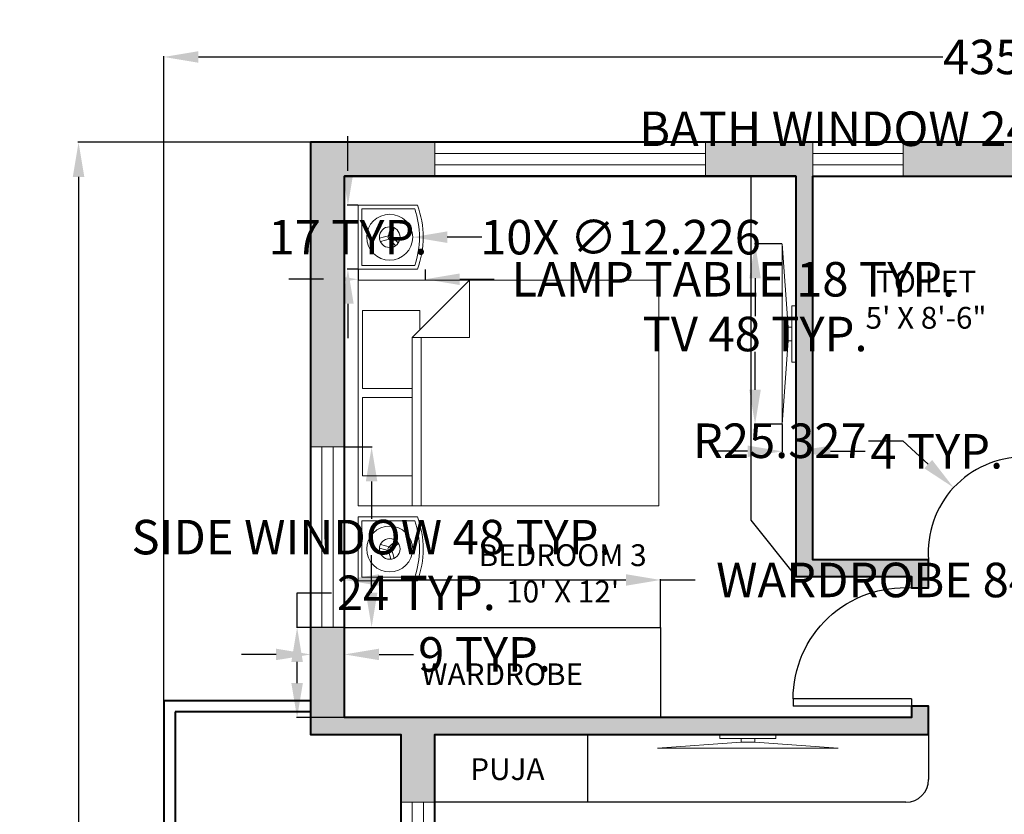
# Model space of a CAD drawing. Units: inches. Extents: x -51 to 563, y -59 to 453.
# Tile 3 of 6: x -51 to 211, y 242 to 453. Entities that reach past the tile are written whole.
import ezdxf

# ---------------------------------------------------------------- set-up
doc = ezdxf.new("R2010")
doc.units = ezdxf.units.IN
doc.header["$MEASUREMENT"] = 0
for name, color, linetype, lineweight in [('A-ANNO-DIMS', 2, 'Continuous', 18), ('A-ANNO-TEXT', 7, 'Continuous', 18), ('A-AREA-IDEN', 7, 'Continuous', 25), ('A-DOOR', 3, 'Continuous', 25), ('A-EQPM', 8, 'Continuous', 18), ('A-FLOR-CASE', 8, 'Continuous', 25), ('A-FURN', 8, 'Continuous', 18), ('A-GLAZ', 4, 'Continuous', 18), ('A-WALL', 7, 'Continuous', 40), ('A-WALL-PATT', 252, 'Continuous', 13)]:
    doc.layers.add(name, color=color, linetype=linetype, lineweight=lineweight)
doc.styles.get("Standard").update_dxf_attribs({"font": 'arial.ttf'})
doc.dimstyles.get("Standard").update_dxf_attribs({"dimtxt": 9.18, "dimasz": 9.18, "dimexe": 0.18, "dimexo": 0.0625, "dimgap": 0.09, "dimtad": 0, "dimtih": 1, "dimtoh": 1, "dimdec": 1, "dimzin": 0, "dimdsep": 46, "dimlunit": 3, "dimtxsty": 'Standard', "dimcen": 0.09, "dimadec": 0, "dimazin": 0, "dimtfac": 1, "dimtdec": 1, "dimtofl": 0, "dimtmove": 0, "dimatfit": 3, "dimfxl": 1, "dimtolj": 1, "dimtzin": 0, "dimarcsym": 0})

# ---------------------------------------------------------------- blocks, each defined once
blk = doc.blocks.new('Bed - Queen')
for p, q in [((0, -80.00003), (0, 0)), ((0, 0), (59.99999, 0)), ((59.99999, 0), (59.99999, -80.00003)), ((7.99999, -1.2), (28.79998, -1.2)), ((7.99999, -14.4), (7.99999, -1.2)), ((28.79998, -1.2), (28.79998, -14.4)), ((31.19999, -1.2), (51.99999, -1.2)), ((31.19999, -14.4), (31.19999, -1.2)), ((51.99999, -1.2), (51.99999, -16.4)), ((0, -14.4), (44.8, -14.4)), ((59.99999, -29.6), (44.8, -14.4)), ((44.8, -14.4), (44.8, -29.6)), ((44.8, -16.8), (0, -16.8)), ((51.99999, -16.4), (46.79936, -16.4)), ((44.8, -29.6), (59.99999, -29.6)), ((59.99999, -80.00003), (0, -80.00003))]:
    blk.add_line(p, q)
blk = doc.blocks.new('WIN-72IN')
for p, q in [((0, 0), (0, 9)), ((72, 0), (72, 9)), ((72, 6), (0, 6)), ((72, 3), (0, 3))]:
    blk.add_line(p, q)
blk = doc.blocks.new('WIN-48IN')
for p, q in [((9, 48), (0, 48)), ((3, 48), (3, 0)), ((6, 48), (6, 0)), ((9, 0), (0, 0))]:
    blk.add_line(p, q)
blk = doc.blocks.new('WIN-24IN')
for p, q in [((0, 0), (0, 9)), ((24, 0), (24, 9)), ((24, 6), (0, 6)), ((24, 3), (0, 3))]:
    blk.add_line(p, q)
blk = doc.blocks.new('DR-SWING-31_5IN')
for p, q in [((0, 2), (31.5, 2)), ((0, 2), (0, 0)), ((31.5, 2), (31.5, 0)), ((0, 0), (31.5, 0))]:
    blk.add_line(p, q)
blk.add_arc((1.94, 2), 29.56, 0, 93.7558)
blk = doc.blocks.new('TV-FLATSCREEN-48IN')
for p, q in [((0, 0), (22.17, 1.61)), ((48, 0), (25.84, 1.61)), ((0, 0), (48, 0))]:
    blk.add_line(p, q)
for points in [[(16.55, 3.67), (31.46, 3.67), (31.46, 2.61), (16.55, 2.61)], [(22.17, 2.61), (25.84, 2.61), (25.84, 1.61), (22.17, 1.61)]]:
    blk.add_lwpolyline(points, close=True)
blk = doc.blocks.new('*U11')
for p, q in [((-1.31, -0.61), (0.61, 1.31)), ((-0.61, -1.31), (1.31, 0.61))]:
    blk.add_line(p, q)
blk = doc.blocks.new('*U12')
at = {"color": 0, "linetype": 'ByBlock', "lineweight": -2, "transparency": 16777216}
for p, rotation in [((276.07, -10.08), 120), ((277.73, -11.74), 239.9999999999999)]:
    blk.add_blockref('*U11', p, dxfattribs=dict(at, rotation=rotation))
blk.add_blockref('*U11', (278.34, -9.47), dxfattribs=at)
blk = doc.blocks.new('TABLE-SIDE-WITH-LAMP')
for points in [[(17.03, 15.79), (17.03, 0), (0, 0), (0, 15.79, -0.18199)], [(16.03, 15.08), (16.03, 1), (1, 1), (1, 15.08, -0.16668)]]:
    blk.add_lwpolyline(points, format="xyb", close=True)
for centre, radius in [((8.51, 8.42), 6.11), ((8.51, 8.42), 2.75), ((8.51, 8.47), 0.5)]:
    blk.add_circle(centre, radius)
blk.add_blockref('*U12', (-268.87, 18.9))
blk = doc.blocks.new('WARDROBE-84X24IN')
for p, q in [((0, 24), (84, 24)), ((84, 24), (84, 0))]:
    blk.add_line(p, q)
blk = doc.blocks.new('*D23')
at = {"layer": 'A-ANNO-DIMS', "color": 0, "lineweight": -2, "transparency": 16777216}
for p, q in [((39.15, 387.04), (39.15, 384.25)), ((57, 387.04), (57, 384.25)), ((29.97, 384.43), (20.79, 384.43)), ((66.18, 384.43), (75.36, 384.43))]:
    blk.add_line(p, q, dxfattribs=at)
at = {"layer": 'A-ANNO-DIMS', "color": 0, "transparency": 16777216}
for points in [[(29.97, 385.96), (29.97, 382.9), (39.15, 384.43)], [(66.18, 385.96), (66.18, 382.9), (57, 384.43)]]:
    blk.add_solid(points, dxfattribs=at)
at = {"layer": 'Defpoints', "color": 0, "transparency": 16777216}
for p in [(39.15, 387.11), (57, 387.11), (57, 384.43)]:
    blk.add_point(p, dxfattribs=at)
at = {"layer": 'A-ANNO-DIMS', "color": 0, "transparency": 16777216, "insert": (138.92, 384.43), "char_height": 9.18, "attachment_point": 5}
blk.add_mtext('\\A1;LAMP TABLE 18 TYP.', dxfattribs=at)
blk = doc.blocks.new('*D24')
at = {"layer": 'A-ANNO-DIMS', "color": 0, "lineweight": -2, "transparency": 16777216}
for p, q in [((36.47, 413.31), (36.47, 422.49)), ((39.08, 404.13), (36.29, 404.13)), ((39.08, 387.11), (36.29, 387.11)), ((36.47, 377.93), (36.47, 368.75))]:
    blk.add_line(p, q, dxfattribs=at)
at = {"layer": 'A-ANNO-DIMS', "color": 0, "transparency": 16777216}
for points in [[(34.94, 413.31), (38, 413.31), (36.47, 404.13)], [(34.94, 377.93), (38, 377.93), (36.47, 387.11)]]:
    blk.add_solid(points, dxfattribs=at)
at = {"layer": 'Defpoints', "color": 0, "transparency": 16777216}
for p in [(39.15, 404.13), (36.47, 387.11), (39.15, 387.11)]:
    blk.add_point(p, dxfattribs=at)
at = {"layer": 'A-ANNO-DIMS', "color": 0, "transparency": 16777216, "insert": (36.47, 395.62), "char_height": 9.18, "attachment_point": 5}
blk.add_mtext('\\A1;17 TYP.', dxfattribs=at)
blk = doc.blocks.new('*D25')
at = {"layer": 'A-ANNO-DIMS', "color": 0, "lineweight": -2, "transparency": 16777216}
for p, q in [((151.82, 393.87), (144.51, 393.87)), ((144.69, 384.69), (144.69, 374.65)), ((144.69, 355.05), (144.69, 365.09)), ((151.82, 345.87), (144.51, 345.87))]:
    blk.add_line(p, q, dxfattribs=at)
at = {"layer": 'A-ANNO-DIMS', "color": 0, "transparency": 16777216}
for points in [[(143.16, 384.69), (146.22, 384.69), (144.69, 393.87)], [(143.16, 355.05), (146.22, 355.05), (144.69, 345.87)]]:
    blk.add_solid(points, dxfattribs=at)
at = {"layer": 'Defpoints', "color": 0, "transparency": 16777216}
for p in [(151.89, 393.87), (144.69, 345.87), (151.89, 345.87)]:
    blk.add_point(p, dxfattribs=at)
at = {"layer": 'A-ANNO-DIMS', "color": 0, "transparency": 16777216, "insert": (144.69, 369.87), "char_height": 9.18, "attachment_point": 5}
blk.add_mtext('\\A1;TV 48 TYP.', dxfattribs=at)
blk = doc.blocks.new('*D26')
at = {"layer": 'A-ANNO-DIMS', "color": 0, "lineweight": -2, "transparency": 16777216}
for p, q in [((151.89, 345.81), (151.89, 338.49)), ((155.56, 345.81), (155.56, 338.49)), ((142.71, 338.67), (133.53, 338.67)), ((164.74, 338.67), (173.92, 338.67))]:
    blk.add_line(p, q, dxfattribs=at)
at = {"layer": 'A-ANNO-DIMS', "color": 0, "transparency": 16777216}
for points in [[(142.71, 340.2), (142.71, 337.14), (151.89, 338.67)], [(164.74, 340.2), (164.74, 337.14), (155.56, 338.67)]]:
    blk.add_solid(points, dxfattribs=at)
at = {"layer": 'Defpoints', "color": 0, "transparency": 16777216}
for p in [(151.89, 345.87), (155.56, 345.87), (155.56, 338.67)]:
    blk.add_point(p, dxfattribs=at)
at = {"layer": 'A-ANNO-DIMS', "color": 0, "transparency": 16777216, "insert": (192.97, 338.67), "char_height": 9.18, "attachment_point": 5}
blk.add_mtext('\\A1;4 TYP.', dxfattribs=at)
blk = doc.blocks.new('*D33')
at = {"layer": 'A-ANNO-DIMS', "color": 0, "lineweight": -2, "transparency": 16777216}
for p, q in [((35.62, 339.85), (42.94, 339.85)), ((42.76, 330.67), (42.76, 320.69)), ((42.76, 301.03), (42.76, 311.01)), ((35.62, 291.85), (42.94, 291.85))]:
    blk.add_line(p, q, dxfattribs=at)
at = {"layer": 'A-ANNO-DIMS', "color": 0, "transparency": 16777216}
for points in [[(41.23, 330.67), (44.29, 330.67), (42.76, 339.85)], [(41.23, 301.03), (44.29, 301.03), (42.76, 291.85)]]:
    blk.add_solid(points, dxfattribs=at)
at = {"layer": 'Defpoints', "color": 0, "transparency": 16777216}
for p in [(35.56, 339.85), (42.76, 339.85), (35.56, 291.85)]:
    blk.add_point(p, dxfattribs=at)
at = {"layer": 'A-ANNO-DIMS', "color": 0, "transparency": 16777216, "insert": (42.76, 315.85), "char_height": 9.18, "attachment_point": 5}
blk.add_mtext('\\A1;SIDE WINDOW 48 TYP.', dxfattribs=at)
blk = doc.blocks.new('*D34')
at = {"layer": 'A-ANNO-DIMS', "color": 0, "lineweight": -2, "transparency": 16777216}
for p, q in [((26.56, 291.79), (26.56, 284.47)), ((35.56, 291.79), (35.56, 284.47)), ((17.38, 284.65), (8.2, 284.65)), ((44.74, 284.65), (53.92, 284.65))]:
    blk.add_line(p, q, dxfattribs=at)
at = {"layer": 'A-ANNO-DIMS', "color": 0, "transparency": 16777216}
for points in [[(17.38, 286.18), (17.38, 283.12), (26.56, 284.65)], [(44.74, 286.18), (44.74, 283.12), (35.56, 284.65)]]:
    blk.add_solid(points, dxfattribs=at)
at = {"layer": 'Defpoints', "color": 0, "transparency": 16777216}
for p in [(26.56, 291.85), (35.56, 291.85), (35.56, 284.65)]:
    blk.add_point(p, dxfattribs=at)
at = {"layer": 'A-ANNO-DIMS', "color": 0, "transparency": 16777216, "insert": (72.78, 284.65), "char_height": 9.18, "attachment_point": 5}
blk.add_mtext('\\A1;9 TYP.', dxfattribs=at)
blk = doc.blocks.new('*D41')
at = {"layer": 'A-ANNO-DIMS', "color": 0, "lineweight": -2, "transparency": 16777216}
for p, q in [((260.56, 424.45), (251.38, 424.45)), ((260.56, 420.91), (260.56, 424.63)), ((275.38, 424.45), (269.74, 424.45)), ((284.56, 420.91), (284.56, 424.63))]:
    blk.add_line(p, q, dxfattribs=at)
at = {"layer": 'A-ANNO-DIMS', "color": 0, "transparency": 16777216}
for points in [[(269.74, 425.98), (269.74, 422.92), (260.56, 424.45)], [(275.38, 425.98), (275.38, 422.92), (284.56, 424.45)]]:
    blk.add_solid(points, dxfattribs=at)
at = {"layer": 'Defpoints', "color": 0, "transparency": 16777216}
for p in [(260.56, 424.45), (260.56, 420.85), (284.56, 420.85)]:
    blk.add_point(p, dxfattribs=at)
at = {"layer": 'A-ANNO-DIMS', "color": 0, "transparency": 16777216, "insert": (180.35, 424.45), "char_height": 9.18, "attachment_point": 5}
blk.add_mtext('\\A1;BATH WINDOW 24 TYP.', dxfattribs=at)
blk = doc.blocks.new('*D47')
at = {"layer": 'A-ANNO-DIMS', "color": 0, "lineweight": -2, "transparency": 16777216}
for p, q in [((35.56, 291.91), (35.56, 304.63)), ((44.74, 304.45), (110.38, 304.45)), ((119.56, 291.91), (119.56, 304.63)), ((119.56, 304.45), (128.74, 304.45))]:
    blk.add_line(p, q, dxfattribs=at)
at = {"layer": 'A-ANNO-DIMS', "color": 0, "transparency": 16777216}
for points in [[(44.74, 305.98), (44.74, 302.92), (35.56, 304.45)], [(110.38, 305.98), (110.38, 302.92), (119.56, 304.45)]]:
    blk.add_solid(points, dxfattribs=at)
at = {"layer": 'Defpoints', "color": 0, "transparency": 16777216}
for p in [(119.56, 304.45), (35.56, 291.85), (119.56, 291.85)]:
    blk.add_point(p, dxfattribs=at)
at = {"layer": 'A-ANNO-DIMS', "color": 0, "transparency": 16777216, "insert": (190.9, 304.45), "char_height": 9.18, "attachment_point": 5}
blk.add_mtext('\\A1;WARDROBE 84 TYP.', dxfattribs=at)
blk = doc.blocks.new('*D48')
at = {"layer": 'A-ANNO-DIMS', "color": 0, "lineweight": -2, "transparency": 16777216}
for p, q in [((22.96, 291.85), (22.96, 301.03)), ((22.96, 301.03), (32.14, 301.03)), ((35.5, 291.85), (22.78, 291.85)), ((22.96, 277.03), (22.96, 282.67)), ((35.5, 267.85), (22.78, 267.85))]:
    blk.add_line(p, q, dxfattribs=at)
at = {"layer": 'A-ANNO-DIMS', "color": 0, "transparency": 16777216}
for points in [[(21.43, 282.67), (24.49, 282.67), (22.96, 291.85)], [(21.43, 277.03), (24.49, 277.03), (22.96, 267.85)]]:
    blk.add_solid(points, dxfattribs=at)
at = {"layer": 'Defpoints', "color": 0, "transparency": 16777216}
for p in [(22.96, 291.85), (35.56, 291.85), (35.56, 267.85)]:
    blk.add_point(p, dxfattribs=at)
at = {"layer": 'A-ANNO-DIMS', "color": 0, "transparency": 16777216, "insert": (54.65, 301.03), "char_height": 9.18, "attachment_point": 5}
blk.add_mtext('\\A1;24 TYP.', dxfattribs=at)
blk = doc.blocks.new('*D65')
at = {"layer": 'A-ANNO-DIMS', "color": 0, "lineweight": -2, "transparency": 16777216}
for p, q in [((-12.44, 272.41), (-12.44, 443.73)), ((-3.26, 443.55), (194.61, 443.55)), ((413.38, 443.55), (215.51, 443.55)), ((422.56, 420.91), (422.56, 443.73))]:
    blk.add_line(p, q, dxfattribs=at)
at = {"layer": 'A-ANNO-DIMS', "color": 0, "transparency": 16777216}
for points in [[(-3.26, 445.08), (-3.26, 442.02), (-12.44, 443.55)], [(413.38, 445.08), (413.38, 442.02), (422.56, 443.55)]]:
    blk.add_solid(points, dxfattribs=at)
at = {"layer": 'Defpoints', "color": 0, "transparency": 16777216}
for p in [(422.56, 443.55), (422.56, 420.85), (-12.44, 272.35)]:
    blk.add_point(p, dxfattribs=at)
at = {"layer": 'A-ANNO-DIMS', "color": 0, "transparency": 16777216, "insert": (205.06, 443.55), "char_height": 9.18, "attachment_point": 5}
blk.add_mtext('\\A1;435', dxfattribs=at)
blk = doc.blocks.new('*D66')
at = {"layer": 'A-ANNO-DIMS', "color": 0, "lineweight": -2, "transparency": 16777216}
for p, q in [((26.5, 420.85), (-35.32, 420.85)), ((-35.14, 411.67), (-35.14, 199.87)), ((-35.14, -21.47), (-35.14, 190.32)), ((26.5, -30.65), (-35.32, -30.65))]:
    blk.add_line(p, q, dxfattribs=at)
at = {"layer": 'A-ANNO-DIMS', "color": 0, "transparency": 16777216}
for points in [[(-36.67, 411.67), (-33.61, 411.67), (-35.14, 420.85)], [(-36.67, -21.47), (-33.61, -21.47), (-35.14, -30.65)]]:
    blk.add_solid(points, dxfattribs=at)
at = {"layer": 'Defpoints', "color": 0, "transparency": 16777216}
for p in [(-35.14, 420.85), (26.56, 420.85), (26.56, -30.65)]:
    blk.add_point(p, dxfattribs=at)
at = {"layer": 'A-ANNO-DIMS', "color": 0, "transparency": 16777216, "insert": (-35.14, 195.1), "char_height": 9.18, "attachment_point": 5}
blk.add_mtext('\\A1;451.5', dxfattribs=at)
blk = doc.blocks.new('*D83')
at = {"layer": 'A-ANNO-DIMS', "color": 0, "lineweight": -2, "transparency": 16777216}
for p, q in [((174.81, 341.48), (183.99, 341.48)), ((183.99, 341.48), (190.73, 335.25)), ((215.97, 311.82), (216.15, 311.82)), ((216.06, 311.73), (216.06, 311.91))]:
    blk.add_line(p, q, dxfattribs=at)
at = {"layer": 'A-ANNO-DIMS', "color": 0, "transparency": 16777216}
blk.add_solid([(191.76, 336.37), (189.69, 334.13), (197.46, 329.02)], dxfattribs=at)
at = {"layer": 'Defpoints', "color": 0, "transparency": 16777216}
for p in [(197.46, 329.02), (216.06, 311.82)]:
    blk.add_point(p, dxfattribs=at)
at = {"layer": 'A-ANNO-DIMS', "color": 0, "transparency": 16777216, "insert": (151.27, 341.48), "char_height": 9.18, "attachment_point": 5}
blk.add_mtext('\\A1;R25.327', dxfattribs=at)
blk = doc.blocks.new('*D98')
at = {"layer": 'A-ANNO-DIMS', "color": 0, "lineweight": -2, "transparency": 16777216}
for p, q in [((47.47, 395.62), (47.65, 395.62)), ((47.56, 395.53), (47.56, 395.71)), ((72.04, 395.62), (62.86, 395.62))]:
    blk.add_line(p, q, dxfattribs=at)
at = {"layer": 'A-ANNO-DIMS', "color": 0, "transparency": 16777216}
blk.add_solid([(62.86, 397.15), (62.86, 394.09), (53.68, 395.62)], dxfattribs=at)
at = {"layer": 'Defpoints', "color": 0, "transparency": 16777216}
for p in [(41.45, 395.62), (53.68, 395.62)]:
    blk.add_point(p, dxfattribs=at)
at = {"layer": 'A-ANNO-DIMS', "color": 0, "transparency": 16777216, "insert": (108.93, 395.62), "char_height": 9.18, "attachment_point": 5}
blk.add_mtext('\\A1;10X ∅12.226', dxfattribs=at)

msp = doc.modelspace()

# ---------------------------------------------------------------- linework, layer by layer
at = {"layer": 'A-DOOR'}
msp.add_arc((216.0584, 311.8209), 25.327, 90, 184.468005, dxfattribs=at)
at = {"layer": 'A-FLOR-CASE'}
for p, q in [((143.5584, 411.8479), (143.5584, 320.3479)), ((143.5584, 320.3479), (155.5584, 305.3479)), ((100.1336, 263.3479), (100.1336, 245.3479)), ((190.8084, 263.3479), (190.8084, 251.3479)), ((180.3084, 245.3479), (59.5584, 245.3479)), ((184.8084, 245.3479), (180.3084, 245.3479))]:
    msp.add_line(p, q, dxfattribs=at)
msp.add_arc((184.8084, 251.3479), 6, 270, 0, dxfattribs=at)
at = {"layer": 'A-GLAZ'}
for p, q in [((50.5584, 245.3479), (59.5584, 245.3479)), ((53.5584, 245.3479), (53.5584, 149.3479)), ((56.5584, 245.3479), (56.5584, 149.3479))]:
    msp.add_line(p, q, dxfattribs=at)
at = {"layer": 'A-WALL'}
for p, q in [((155.5584, 411.8479), (35.5584, 411.8479)), ((-9.4416, 269.3479), (-9.4416, 125.3479)), ((26.5584, 269.3479), (-9.4416, 269.3479))]:
    msp.add_line(p, q, dxfattribs=at)
for points in [[(422.5584, 420.8479), (26.5584, 420.8479), (26.5584, 267.8479), (26.5584, 263.3479), (35.5584, 263.3479), (50.5584, 263.3479), (50.5584, 131.3479), (35.5584, 131.3479), (26.5584, 131.3479), (26.5584, 126.8479), (26.5584, 0.8479), (26.5584, -30.6521), (35.5584, -30.6521), (284.5584, -30.6521)], [(59.5584, 131.3479), (59.5584, 263.3479), (186.3084, 263.3479), (190.8084, 263.3479), (190.8084, 267.8479), (190.8084, 270.8479), (186.3084, 270.8479), (186.3084, 267.8479), (160.0584, 267.8479), (155.5584, 267.8479), (35.5584, 267.8479), (35.5584, 411.8479), (155.5584, 411.8479), (155.5584, 305.3479), (160.0584, 305.3479), (186.3084, 305.3479), (186.3084, 302.3479), (190.8084, 302.3479), (190.8084, 305.3479), (190.8084, 309.8479), (160.0584, 309.8479), (160.0584, 411.8479), (220.0584, 411.8479)], [(26.5584, 272.3479), (-9.4416, 272.3479), (-12.4416, 272.3479), (-12.4416, 267.8479), (-12.4416, 126.8479), (-12.4416, 122.3479), (-9.4416, 122.3479), (26.5584, 122.3479)]]:
    msp.add_lwpolyline(points, dxfattribs=at)
at = {"layer": 'A-WALL-PATT'}
for points in [[(59.5584, 411.8479), (59.5584, 420.8479), (35.5584, 411.8479), (26.5584, 420.8479)], [(35.5584, 411.8479), (26.5584, 420.8479), (35.5584, 339.8479), (26.5584, 339.8479)], [(155.5584, 411.8479), (160.0584, 420.8479), (131.5584, 411.8479), (131.5584, 420.8479)], [(155.5584, 305.3479), (160.0584, 309.8479), (155.5584, 411.8479), (160.0584, 420.8479)], [(184.0584, 420.8479), (184.0584, 411.8479), (260.5584, 420.8479), (260.5584, 411.8479)], [(186.3084, 305.3479), (190.8084, 309.8479), (155.5584, 305.3479), (160.0584, 309.8479)], [(186.3084, 302.3479), (190.8084, 302.3479), (186.3084, 305.3479), (190.8084, 309.8479)], [(26.5584, 291.8479), (35.5584, 291.8479), (26.5584, 263.3479), (35.5584, 267.8479)], [(190.8084, 263.3479), (186.3084, 267.8479), (190.8084, 270.8479), (186.3084, 270.8479)], [(26.5584, 263.3479), (35.5584, 267.8479), (190.8084, 263.3479), (186.3084, 267.8479)], [(50.5584, 263.3479), (59.5584, 263.3479), (50.5584, 245.3479), (59.5584, 245.3479)]]:
    msp.add_solid(points, dxfattribs=at)

# ---------------------------------------------------------------- block references
at = {"layer": 'A-DOOR', "extrusion": (0, 0, -1), "zscale": -1}
msp.add_blockref('DR-SWING-31_5IN', (-186.3087, 270.848), dxfattribs=at)
at = {"layer": 'A-EQPM', "rotation": 270.0000000000002}
msp.add_blockref('TV-FLATSCREEN-48IN', (151.8855, 393.8684), dxfattribs=at)
at = {"layer": 'A-EQPM'}
msp.add_blockref('TV-FLATSCREEN-48IN', (118.7846, 259.675), dxfattribs=at)
at = {"layer": 'A-FLOR-CASE'}
msp.add_blockref('WARDROBE-84X24IN', (35.558, 267.848), dxfattribs=at)
at = {"layer": 'A-FURN'}
for name, p, rotation in [('TABLE-SIDE-WITH-LAMP', (39.1458, 404.1317), 270.0000000000001), ('Bed - Queen', (39.1462, 324.1581), 89.99999999999999)]:
    msp.add_blockref(name, p, dxfattribs=dict(at, rotation=rotation))
at = {"layer": 'A-FURN', "extrusion": (0, 0, -1), "zscale": -1, "rotation": 89.99999999999989}
msp.add_blockref('TABLE-SIDE-WITH-LAMP', (-39.1458, 304.1845), dxfattribs=at)
at = {"layer": 'A-GLAZ'}
for name, p in [('WIN-72IN', (59.558, 411.848)), ('WIN-24IN', (160.058, 411.848)), ('WIN-48IN', (26.558, 291.848))]:
    msp.add_blockref(name, p, dxfattribs=at)

# ---------------------------------------------------------------- texts
at = {"layer": 'A-ANNO-TEXT', "insert": (52.6952, 282.2738), "char_height": 5.8, "attachment_point": 1}
msp.add_mtext_dynamic_manual_height_columns('\\pxqc;WARDROBE', width=49.588896, gutter_width=1, heights=[0], dxfattribs=at)
at = {"layer": 'A-AREA-IDEN', "char_height": 5.8, "attachment_point": 1}
for s, width, insert in [('\\pxqc;TOILET\\P5\' X 8\'-6"', 49.588896, (165.3516, 386.7482)), ("\\pxqc;BEDROOM 3\\P10' X 12'", 49.588896, (68.7462, 313.9383)), ('\\pxqc;PUJA', 21.967762, (67.87, 257.0438))]:
    msp.add_mtext_dynamic_manual_height_columns(s, width=width, gutter_width=1, heights=[0], dxfattribs=dict(at, insert=insert))

# ---------------------------------------------------------------- dimensions: what is measured, and where the dimension line sits
at = {"layer": 'A-ANNO-DIMS'}
for base, p1, p2, angle, text, picture, middle in [((260.5584, 424.4479), (284.5584, 420.8479), (260.5584, 420.8479), 180, 'BATH WINDOW <> TYP.', '*D41', (180.35, 424.4479)), ((36.4686, 387.1065), (39.1462, 404.1319), (39.1462, 387.1065), 270, '<> TYP.', '*D24', (36.4686, 395.6192)), ((56.9966, 384.429), (39.1462, 387.1065), (56.9966, 387.1065), 0, 'LAMP TABLE <> TYP.', '*D23', (138.9238, 384.429)), ((144.6851, 345.8688), (151.8851, 393.8688), (151.8851, 345.8688), 270, 'TV <> TYP.', '*D25', (144.6851, 369.8688)), ((42.7584, 339.8479), (35.5584, 291.8479), (35.5584, 339.8479), 90, 'SIDE WINDOW <> TYP.', '*D33', (42.7584, 315.8479)), ((22.9584, 291.8479), (35.5584, 267.8479), (35.5584, 291.8479), 90, '<> TYP.', '*D48', (54.6492, 301.0279))]:
    dim = msp.add_linear_dim(base=base, p1=p1, p2=p2, angle=angle, text=text, dimstyle='Standard', override={"dimdec": 0, "dimlfac": 1, "dimrnd": 0, "dimzin": 0, "dimdsep": 46, "dimlunit": 2}, dxfattribs=at)
    dim.commit()
    dim.dimension.update_dxf_attribs({"geometry": picture, "text_midpoint": middle})
dim = msp.add_linear_dim(base=(422.5584, 443.5479), p1=(-12.4416, 272.3479), p2=(422.5584, 420.8479), dimstyle='Standard', override={"dimdec": 0, "dimlfac": 1, "dimrnd": 0, "dimzin": 0, "dimdsep": 46, "dimlunit": 2}, dxfattribs=at)
dim.commit()
dim.dimension.update_dxf_attribs({"geometry": '*D65', "text_midpoint": (205.0584, 443.5479)})
dim = msp.add_linear_dim(base=(-35.1416, 420.8479), p1=(26.5584, -30.6521), p2=(26.5584, 420.8479), angle=90, dimstyle='Standard', override={"dimdec": 1, "dimlfac": 1, "dimrnd": 0, "dimzin": 0, "dimdsep": 46, "dimlunit": 2}, dxfattribs=at)
dim.commit()
dim.dimension.update_dxf_attribs({"geometry": '*D66', "text_midpoint": (-35.1416, 195.0979)})
dim = msp.add_diameter_dim_2p(p1=(41.4516, 395.6194), p2=(53.6777, 395.619), text='10X <>', dimstyle='Standard', override={"dimdec": 3, "dimlfac": 1, "dimrnd": 0, "dimzin": 0, "dimdsep": 46, "dimlunit": 2}, dxfattribs=at)
dim.commit()
dim.dimension.update_dxf_attribs({"geometry": '*D98', "text_midpoint": (72.0377, 395.6183), "dimtype": 163})
for base, p1, p2, text, picture, middle in [((155.5584, 338.6688), (151.8851, 345.8688), (155.5584, 345.8688), '<> TYP.', '*D26', (192.9695, 338.6688)), ((119.5584, 304.4479), (35.5584, 291.8479), (119.5584, 291.8479), 'WARDROBE <> TYP.', '*D47', (190.903, 304.4479)), ((35.5584, 284.6479), (26.5584, 291.8479), (35.5584, 291.8479), '<> TYP.', '*D34', (72.7848, 284.6479))]:
    dim = msp.add_linear_dim(base=base, p1=p1, p2=p2, text=text, dimstyle='Standard', override={"dimdec": 0, "dimlfac": 1, "dimrnd": 0, "dimzin": 0, "dimdsep": 46, "dimlunit": 2}, dxfattribs=at)
    dim.commit()
    dim.dimension.update_dxf_attribs({"geometry": picture, "text_midpoint": middle})
dim = msp.add_radius_dim(center=(216.0584, 311.8209), mpoint=(197.465, 329.018), dimstyle='Standard', override={"dimdec": 3, "dimlfac": 1, "dimrnd": 0, "dimzin": 0, "dimdsep": 46, "dimlunit": 2}, dxfattribs=at)
dim.commit()
dim.dimension.update_dxf_attribs({"geometry": '*D83', "text_midpoint": (151.2684, 341.4845)})

doc.saveas('drawing.dxf')
